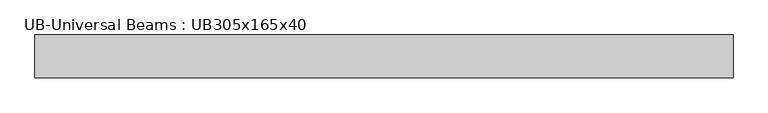
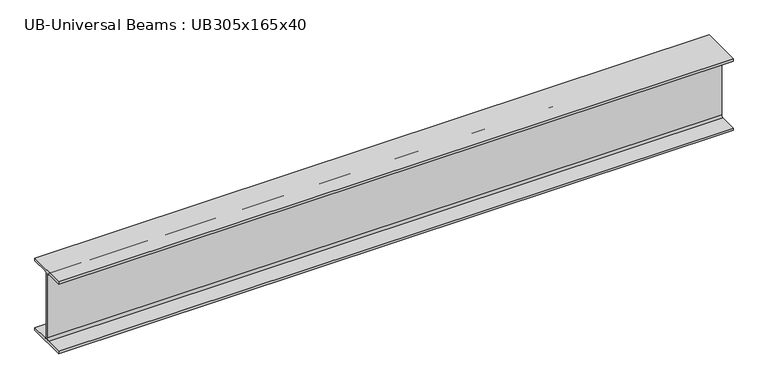
"""IFC4 building model written with IfcOpenShell, lengths in millimetres: beam geometry, UB-Universal Beams : UB305x165x40."""

from ifc_helpers import new_model, si_unit, point, frame, frame_2d, origin, place, context, project, spatial, polyline, circle_curve, trimmed, segment, composite_curve, outline, extrude, source, transform, mapped, element, save


def ub_universal_beams_ub305x165x40_ffb14e35(model_context):
    return source(origin(), model_context, "Body", "SweptSolid", [
        extrude(outline(composite_curve([segment(polyline([(82.5, -141.5), (82.5, -151.7), (-82.5, -151.7), (-82.5, -141.5), (-11.9, -141.5)]), True, "CONTINUOUS"), segment(trimmed(circle_curve(frame_2d((-11.9, -132.6)), 8.9), [point((-11.9, -141.5))], [point((-3.0, -132.6))], True, "CARTESIAN"), True, "CONTINUOUS"), segment(polyline([(-3.0, -132.6), (-3.0, 132.6)]), True, "CONTINUOUS"), segment(trimmed(circle_curve(frame_2d((-11.9, 132.6)), 8.9), [point((-3.0, 132.6))], [point((-11.9, 141.5))], True, "CARTESIAN"), True, "CONTINUOUS"), segment(polyline([(-11.9, 141.5), (-82.5, 141.5), (-82.5, 151.7), (82.5, 151.7), (82.5, 141.5), (11.9, 141.5)]), True, "CONTINUOUS"), segment(trimmed(circle_curve(frame_2d((11.9, 132.6)), 8.9), [point((11.9, 141.5))], [point((3.0, 132.6))], True, "CARTESIAN"), True, "CONTINUOUS"), segment(polyline([(3.0, 132.6), (3.0, -132.6)]), True, "CONTINUOUS"), segment(trimmed(circle_curve(frame_2d((11.9, -132.6)), 8.9), [point((3.0, -132.6))], [point((11.9, -141.5))], True, "CARTESIAN"), True, "CONTINUOUS"), segment(polyline([(11.9, -141.5), (82.5, -141.5)]), True, "CONTINUOUS")], self_intersect=False)), frame((-1337.3, 0.0, 0.0), z_axis=(1.0, 0.0, 0.0), x_axis=(0.0, 1.0, 0.0)), (0.0, 0.0, 1.0), 2692.1),
    ])


if __name__ == "__main__":
    model = new_model("IFC4")
    model_context = context("Model", 3, world=origin())
    ifc_project = project(units=[si_unit("LENGTHUNIT", "METRE", prefix="MILLI")], contexts=[model_context])
    site = spatial("IfcSite", under=ifc_project)
    building = spatial("IfcBuilding", under=site)
    placement = place(None, origin())
    ub_universal_beams_ub305x165x40_shape = ub_universal_beams_ub305x165x40_ffb14e35(model_context)
    element("IfcBeam", 1, ObjectType="UB-Universal Beams : UB305x165x40", at=placement, inside=building, context=model_context, shape_type="MappedRepresentation", body=[
        mapped(ub_universal_beams_ub305x165x40_shape, transform((0.0, 0.0, 0.0), x_axis=(1.0, 0.0, 0.0), y_axis=(0.0, 1.0, 0.0), z_axis=(0.0, 0.0, 1.0))),
    ])
    save(model, "model.ifc")

# Revit data of these elements
# Type "UB-Universal Beams : UB305x165x40"
#   Section Name Key = "UB305X165X40"
#   Width = 16.5 cm
#   Web Thickness = 0.6 cm
#   Web Fillet = 0.89 cm
#   Warping Constant = 164000.0 cm⁶
#   Torsional Moment of Inertia = 14.70 cm⁴
#   Section Area = 51.3 cm²
#   Plastic Modulus weak axis = 142.0 cm³
#   Plastic Modulus strong axis = 623.0 cm³
#   Nominal Weight = 40.2999 kgf/m
#   Moment of Inertia weak axis = 764.00 cm⁴
#   Moment of Inertia strong axis = 8503.00 cm⁴
#   Height = 30.34 cm
#   Flange Thickness = 1.02 cm
#   Elastic Modulus weak axis = 92.6 cm³
#   Elastic Modulus strong axis = 560.0 cm³
#   Centroid Vertical = 15.17 cm
#   Centroid Horizontal = 8.25 cm
#   Bolt Spacing = 9.0 cm
#   Length [instance default] = 1.5 m
#   Structural Material [instance default] = Metal - Steel 43-275
#   Type Comments = ""
#   Assembly Code = ""
# Element 1 (IfcBeam, "UB-Universal Beams : UB305x165x40")
#   Materials on its faces: "Metal - Steel 43-275"
# Materials
#   "Metal - Steel 43-275": class "Metal", colour RGB 247 247 247, transparency 0, Cost = 0
